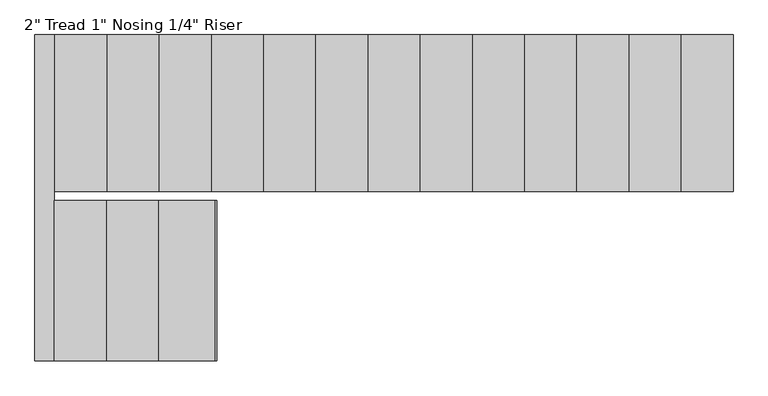
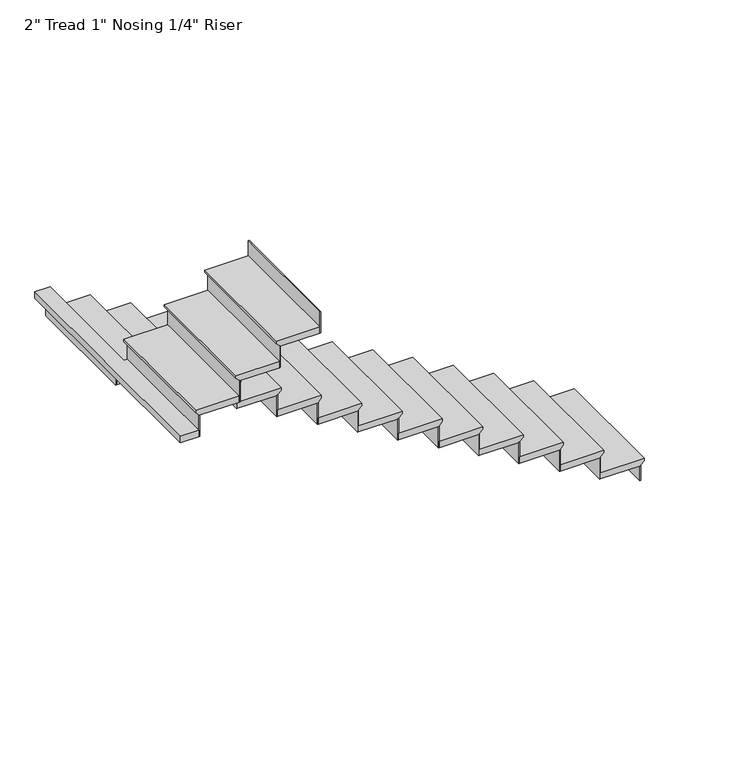
"""IFC4 building model written with IfcOpenShell, lengths in millimetres: stair flight geometry."""

from ifc_helpers import new_model, si_unit, origin, place, context, project, spatial, faceted_brep, source, transform, mapped, element, save


def stair_flight_af090c4c(model_context):
    return source(origin(), model_context, "Body", "Brep", [
        faceted_brep([(6794.5, 11386.0372886, 6246.2833333), (6794.5, 11386.0372886, 6265.3333333), (6794.5, 10471.6372886, 6265.3333333), (6794.5, 10471.6372886, 6246.2833333), (6769.1, 11386.0372886, 6220.8833333), (6769.1, 10471.6372886, 6220.8833333), (6464.3, 11386.0372886, 6265.3333333), (6464.3, 10471.6372886, 6265.3333333), (6769.1, 10471.6372886, 6214.5333333), (6464.3, 10471.6372886, 6214.5333333), (6464.3, 11386.0372886, 6214.5333333), (6769.1, 11386.0372886, 6214.5333333)], [[[0, 1, 2, 3]], [[4, 0, 3, 5]], [[2, 1, 6, 7]], [[8, 9, 10, 11]], [[2, 7, 9, 8, 5, 3]], [[8, 11, 4, 5]], [[6, 1, 0, 4, 11, 10]], [[7, 6, 10, 9]]]),
        faceted_brep([(6769.1, 11386.0372886, 6214.5333333), (6769.1, 11386.0372886, 6096.0), (6762.75, 11386.0372886, 6096.0), (6762.75, 11386.0372886, 6214.5333333), (6769.1, 10471.6372886, 6214.5333333), (6762.75, 10471.6372886, 6214.5333333), (6762.75, 10471.6372886, 6096.0), (6769.1, 10471.6372886, 6096.0)], [[[0, 1, 2, 3]], [[4, 5, 6, 7]], [[1, 0, 4, 7]], [[2, 1, 7, 6]], [[3, 2, 6, 5]], [[0, 3, 5, 4]]]),
        faceted_brep([(6464.3, 11386.0372886, 6383.8666667), (6464.3, 11386.0372886, 6214.5333333), (6457.95, 11386.0372886, 6214.5333333), (6457.95, 11386.0372886, 6383.8666667), (6464.3, 10471.6372886, 6383.8666667), (6457.95, 10471.6372886, 6383.8666667), (6457.95, 10471.6372886, 6214.5333333), (6464.3, 10471.6372886, 6214.5333333)], [[[0, 1, 2, 3]], [[4, 5, 6, 7]], [[1, 0, 4, 7]], [[2, 1, 7, 6]], [[3, 2, 6, 5]], [[0, 3, 5, 4]]]),
        faceted_brep([(6489.7, 10471.6372886, 6434.6666667), (6489.7, 11386.0372886, 6434.6666667), (6159.5, 11386.0372886, 6434.6666667), (6159.5, 10471.6372886, 6434.6666667), (6464.3, 10471.6372886, 6383.8666667), (6159.5, 10471.6372886, 6383.8666667), (6159.5, 11386.0372886, 6383.8666667), (6464.3, 11386.0372886, 6383.8666667), (6464.3, 10471.6372886, 6390.2166667), (6489.7, 10471.6372886, 6415.6166667), (6464.3, 11386.0372886, 6390.2166667), (6489.7, 11386.0372886, 6415.6166667)], [[[0, 1, 2, 3]], [[4, 5, 6, 7]], [[0, 3, 5, 4, 8, 9]], [[4, 7, 10, 8]], [[2, 1, 11, 10, 7, 6]], [[3, 2, 6, 5]], [[11, 1, 0, 9]], [[10, 11, 9, 8]]]),
        faceted_brep([(6159.5, 11386.0372886, 6553.2), (6159.5, 11386.0372886, 6383.8666667), (6153.15, 11386.0372886, 6383.8666667), (6153.15, 11386.0372886, 6553.2), (6159.5, 10471.6372886, 6553.2), (6153.15, 10471.6372886, 6553.2), (6153.15, 10471.6372886, 6383.8666667), (6159.5, 10471.6372886, 6383.8666667)], [[[0, 1, 2, 3]], [[4, 5, 6, 7]], [[1, 0, 4, 7]], [[2, 1, 7, 6]], [[3, 2, 6, 5]], [[0, 3, 5, 4]]]),
        faceted_brep([(6184.9, 10471.6372886, 6604.0), (6184.9, 11386.0372886, 6604.0), (5854.7, 11386.0372886, 6604.0), (5854.7, 10471.6372886, 6604.0), (6159.5, 10471.6372886, 6553.2), (5854.7, 10471.6372886, 6553.2), (5854.7, 11386.0372886, 6553.2), (6159.5, 11386.0372886, 6553.2), (6159.5, 10471.6372886, 6559.55), (6184.9, 10471.6372886, 6584.95), (6159.5, 11386.0372886, 6559.55), (6184.9, 11386.0372886, 6584.95)], [[[0, 1, 2, 3]], [[4, 5, 6, 7]], [[0, 3, 5, 4, 8, 9]], [[4, 7, 10, 8]], [[2, 1, 11, 10, 7, 6]], [[3, 2, 6, 5]], [[11, 1, 0, 9]], [[10, 11, 9, 8]]]),
        faceted_brep([(5854.7, 11386.0372886, 6722.5333333), (5854.7, 11386.0372886, 6553.2), (5848.35, 11386.0372886, 6553.2), (5848.35, 11386.0372886, 6722.5333333), (5854.7, 10471.6372886, 6722.5333333), (5848.35, 10471.6372886, 6722.5333333), (5848.35, 10471.6372886, 6553.2), (5854.7, 10471.6372886, 6553.2)], [[[0, 1, 2, 3]], [[4, 5, 6, 7]], [[1, 0, 4, 7]], [[2, 1, 7, 6]], [[3, 2, 6, 5]], [[0, 3, 5, 4]]]),
        faceted_brep([(5880.1, 10471.6372886, 6773.3333333), (5880.1, 11386.0372886, 6773.3333333), (5549.9, 11386.0372886, 6773.3333333), (5549.9, 10471.6372886, 6773.3333333), (5854.7, 10471.6372886, 6722.5333333), (5549.9, 10471.6372886, 6722.5333333), (5549.9, 11386.0372886, 6722.5333333), (5854.7, 11386.0372886, 6722.5333333), (5854.7, 10471.6372886, 6728.8833333), (5880.1, 10471.6372886, 6754.2833333), (5854.7, 11386.0372886, 6728.8833333), (5880.1, 11386.0372886, 6754.2833333)], [[[0, 1, 2, 3]], [[4, 5, 6, 7]], [[0, 3, 5, 4, 8, 9]], [[4, 7, 10, 8]], [[2, 1, 11, 10, 7, 6]], [[3, 2, 6, 5]], [[11, 1, 0, 9]], [[10, 11, 9, 8]]]),
        faceted_brep([(5549.9, 11386.0372886, 6891.8666667), (5549.9, 11386.0372886, 6722.5333333), (5543.55, 11386.0372886, 6722.5333333), (5543.55, 11386.0372886, 6891.8666667), (5549.9, 10471.6372886, 6891.8666667), (5543.55, 10471.6372886, 6891.8666667), (5543.55, 10471.6372886, 6722.5333333), (5549.9, 10471.6372886, 6722.5333333)], [[[0, 1, 2, 3]], [[4, 5, 6, 7]], [[1, 0, 4, 7]], [[2, 1, 7, 6]], [[3, 2, 6, 5]], [[0, 3, 5, 4]]]),
        faceted_brep([(5575.3, 10471.6372886, 6942.6666667), (5575.3, 11386.0372886, 6942.6666667), (5245.1, 11386.0372886, 6942.6666667), (5245.1, 10471.6372886, 6942.6666667), (5549.9, 10471.6372886, 6891.8666667), (5245.1, 10471.6372886, 6891.8666667), (5245.1, 11386.0372886, 6891.8666667), (5549.9, 11386.0372886, 6891.8666667), (5549.9, 10471.6372886, 6898.2166667), (5575.3, 10471.6372886, 6923.6166667), (5549.9, 11386.0372886, 6898.2166667), (5575.3, 11386.0372886, 6923.6166667)], [[[0, 1, 2, 3]], [[4, 5, 6, 7]], [[0, 3, 5, 4, 8, 9]], [[4, 7, 10, 8]], [[2, 1, 11, 10, 7, 6]], [[3, 2, 6, 5]], [[11, 1, 0, 9]], [[10, 11, 9, 8]]]),
        faceted_brep([(5245.1, 11386.0372886, 7061.2), (5245.1, 11386.0372886, 6891.8666667), (5238.75, 11386.0372886, 6891.8666667), (5238.75, 11386.0372886, 7061.2), (5245.1, 10471.6372886, 7061.2), (5238.75, 10471.6372886, 7061.2), (5238.75, 10471.6372886, 6891.8666667), (5245.1, 10471.6372886, 6891.8666667)], [[[0, 1, 2, 3]], [[4, 5, 6, 7]], [[1, 0, 4, 7]], [[2, 1, 7, 6]], [[3, 2, 6, 5]], [[0, 3, 5, 4]]]),
        faceted_brep([(5270.5, 10471.6372886, 7112.0), (5270.5, 11386.0372886, 7112.0), (4940.3, 11386.0372886, 7112.0), (4940.3, 10471.6372886, 7112.0), (5245.1, 10471.6372886, 7061.2), (4940.3, 10471.6372886, 7061.2), (4940.3, 11386.0372886, 7061.2), (5245.1, 11386.0372886, 7061.2), (5245.1, 10471.6372886, 7067.55), (5270.5, 10471.6372886, 7092.95), (5245.1, 11386.0372886, 7067.55), (5270.5, 11386.0372886, 7092.95)], [[[0, 1, 2, 3]], [[4, 5, 6, 7]], [[0, 3, 5, 4, 8, 9]], [[4, 7, 10, 8]], [[2, 1, 11, 10, 7, 6]], [[3, 2, 6, 5]], [[11, 1, 0, 9]], [[10, 11, 9, 8]]]),
        faceted_brep([(4940.3, 11386.0372886, 7230.5333333), (4940.3, 11386.0372886, 7061.2), (4933.95, 11386.0372886, 7061.2), (4933.95, 11386.0372886, 7230.5333333), (4940.3, 10471.6372886, 7230.5333333), (4933.95, 10471.6372886, 7230.5333333), (4933.95, 10471.6372886, 7061.2), (4940.3, 10471.6372886, 7061.2)], [[[0, 1, 2, 3]], [[4, 5, 6, 7]], [[1, 0, 4, 7]], [[2, 1, 7, 6]], [[3, 2, 6, 5]], [[0, 3, 5, 4]]]),
        faceted_brep([(4965.7, 10471.6372886, 7281.3333333), (4965.7, 11386.0372886, 7281.3333333), (4635.5, 11386.0372886, 7281.3333333), (4635.5, 10471.6372886, 7281.3333333), (4940.3, 10471.6372886, 7230.5333333), (4635.5, 10471.6372886, 7230.5333333), (4635.5, 11386.0372886, 7230.5333333), (4940.3, 11386.0372886, 7230.5333333), (4940.3, 10471.6372886, 7236.8833333), (4965.7, 10471.6372886, 7262.2833333), (4940.3, 11386.0372886, 7236.8833333), (4965.7, 11386.0372886, 7262.2833333)], [[[0, 1, 2, 3]], [[4, 5, 6, 7]], [[0, 3, 5, 4, 8, 9]], [[4, 7, 10, 8]], [[2, 1, 11, 10, 7, 6]], [[3, 2, 6, 5]], [[11, 1, 0, 9]], [[10, 11, 9, 8]]]),
        faceted_brep([(4635.5, 11386.0372886, 7399.8666667), (4635.5, 11386.0372886, 7230.5333333), (4629.15, 11386.0372886, 7230.5333333), (4629.15, 11386.0372886, 7399.8666667), (4635.5, 10471.6372886, 7399.8666667), (4629.15, 10471.6372886, 7399.8666667), (4629.15, 10471.6372886, 7230.5333333), (4635.5, 10471.6372886, 7230.5333333)], [[[0, 1, 2, 3]], [[4, 5, 6, 7]], [[1, 0, 4, 7]], [[2, 1, 7, 6]], [[3, 2, 6, 5]], [[0, 3, 5, 4]]]),
        faceted_brep([(4660.9, 10471.6372886, 7450.6666667), (4660.9, 11386.0372886, 7450.6666667), (4330.7, 11386.0372886, 7450.6666667), (4330.7, 10471.6372886, 7450.6666667), (4635.5, 10471.6372886, 7399.8666667), (4330.7, 10471.6372886, 7399.8666667), (4330.7, 11386.0372886, 7399.8666667), (4635.5, 11386.0372886, 7399.8666667), (4635.5, 10471.6372886, 7406.2166667), (4660.9, 10471.6372886, 7431.6166667), (4635.5, 11386.0372886, 7406.2166667), (4660.9, 11386.0372886, 7431.6166667)], [[[0, 1, 2, 3]], [[4, 5, 6, 7]], [[0, 3, 5, 4, 8, 9]], [[4, 7, 10, 8]], [[2, 1, 11, 10, 7, 6]], [[3, 2, 6, 5]], [[11, 1, 0, 9]], [[10, 11, 9, 8]]]),
        faceted_brep([(4330.7, 11386.0372886, 7569.2), (4330.7, 11386.0372886, 7399.8666667), (4324.35, 11386.0372886, 7399.8666667), (4324.35, 11386.0372886, 7569.2), (4330.7, 10471.6372886, 7569.2), (4324.35, 10471.6372886, 7569.2), (4324.35, 10471.6372886, 7399.8666667), (4330.7, 10471.6372886, 7399.8666667)], [[[0, 1, 2, 3]], [[4, 5, 6, 7]], [[1, 0, 4, 7]], [[2, 1, 7, 6]], [[3, 2, 6, 5]], [[0, 3, 5, 4]]]),
        faceted_brep([(4356.1, 10471.6372886, 7620.0), (4356.1, 11386.0372886, 7620.0), (4025.9, 11386.0372886, 7620.0), (4025.9, 10471.6372886, 7620.0), (4330.7, 10471.6372886, 7569.2), (4025.9, 10471.6372886, 7569.2), (4025.9, 11386.0372886, 7569.2), (4330.7, 11386.0372886, 7569.2), (4330.7, 10471.6372886, 7575.55), (4356.1, 10471.6372886, 7600.95), (4330.7, 11386.0372886, 7575.55), (4356.1, 11386.0372886, 7600.95)], [[[0, 1, 2, 3]], [[4, 5, 6, 7]], [[0, 3, 5, 4, 8, 9]], [[4, 7, 10, 8]], [[2, 1, 11, 10, 7, 6]], [[3, 2, 6, 5]], [[11, 1, 0, 9]], [[10, 11, 9, 8]]]),
        faceted_brep([(4025.9, 11386.0372886, 7738.5333333), (4025.9, 11386.0372886, 7569.2), (4019.55, 11386.0372886, 7569.2), (4019.55, 11386.0372886, 7738.5333333), (4025.9, 10471.6372886, 7738.5333333), (4019.55, 10471.6372886, 7738.5333333), (4019.55, 10471.6372886, 7569.2), (4025.9, 10471.6372886, 7569.2)], [[[0, 1, 2, 3]], [[4, 5, 6, 7]], [[1, 0, 4, 7]], [[2, 1, 7, 6]], [[3, 2, 6, 5]], [[0, 3, 5, 4]]]),
        faceted_brep([(4051.3, 10471.6372886, 7789.3333333), (4051.3, 11386.0372886, 7789.3333333), (3721.1, 11386.0372886, 7789.3333333), (3721.1, 10471.6372886, 7789.3333333), (4025.9, 10471.6372886, 7738.5333333), (3721.1, 10471.6372886, 7738.5333333), (3721.1, 11386.0372886, 7738.5333333), (4025.9, 11386.0372886, 7738.5333333), (4025.9, 10471.6372886, 7744.8833333), (4051.3, 10471.6372886, 7770.2833333), (4025.9, 11386.0372886, 7744.8833333), (4051.3, 11386.0372886, 7770.2833333)], [[[0, 1, 2, 3]], [[4, 5, 6, 7]], [[0, 3, 5, 4, 8, 9]], [[4, 7, 10, 8]], [[2, 1, 11, 10, 7, 6]], [[3, 2, 6, 5]], [[11, 1, 0, 9]], [[10, 11, 9, 8]]]),
        faceted_brep([(3721.1, 11386.0372886, 7907.8666667), (3721.1, 11386.0372886, 7738.5333333), (3714.75, 11386.0372886, 7738.5333333), (3714.75, 11386.0372886, 7907.8666667), (3721.1, 10471.6372886, 7907.8666667), (3714.75, 10471.6372886, 7907.8666667), (3714.75, 10471.6372886, 7738.5333333), (3721.1, 10471.6372886, 7738.5333333)], [[[0, 1, 2, 3]], [[4, 5, 6, 7]], [[1, 0, 4, 7]], [[2, 1, 7, 6]], [[3, 2, 6, 5]], [[0, 3, 5, 4]]]),
        faceted_brep([(3746.5, 10471.6372886, 7958.6666667), (3746.5, 11386.0372886, 7958.6666667), (3416.3, 11386.0372886, 7958.6666667), (3416.3, 10471.6372886, 7958.6666667), (3721.1, 10471.6372886, 7907.8666667), (3416.3, 10471.6372886, 7907.8666667), (3416.3, 11386.0372886, 7907.8666667), (3721.1, 11386.0372886, 7907.8666667), (3721.1, 10471.6372886, 7914.2166667), (3746.5, 10471.6372886, 7939.6166667), (3721.1, 11386.0372886, 7914.2166667), (3746.5, 11386.0372886, 7939.6166667)], [[[0, 1, 2, 3]], [[4, 5, 6, 7]], [[0, 3, 5, 4, 8, 9]], [[4, 7, 10, 8]], [[2, 1, 11, 10, 7, 6]], [[3, 2, 6, 5]], [[11, 1, 0, 9]], [[10, 11, 9, 8]]]),
        faceted_brep([(3416.3, 11386.0372886, 8077.2), (3416.3, 11386.0372886, 7907.8666667), (3409.95, 11386.0372886, 7907.8666667), (3409.95, 11386.0372886, 8077.2), (3416.3, 10471.6372886, 8077.2), (3409.95, 10471.6372886, 8077.2), (3409.95, 10471.6372886, 7907.8666667), (3416.3, 10471.6372886, 7907.8666667)], [[[0, 1, 2, 3]], [[4, 5, 6, 7]], [[1, 0, 4, 7]], [[2, 1, 7, 6]], [[3, 2, 6, 5]], [[0, 3, 5, 4]]]),
        faceted_brep([(3441.7, 10471.6372886, 8128.0), (3441.7, 11386.0372886, 8128.0), (3111.5, 11386.0372886, 8128.0), (3111.5, 10471.6372886, 8128.0), (3416.3, 10471.6372886, 8077.2), (3111.5, 10471.6372886, 8077.2), (3111.5, 11386.0372886, 8077.2), (3416.3, 11386.0372886, 8077.2), (3416.3, 10471.6372886, 8083.55), (3441.7, 10471.6372886, 8108.95), (3416.3, 11386.0372886, 8083.55), (3441.7, 11386.0372886, 8108.95)], [[[0, 1, 2, 3]], [[4, 5, 6, 7]], [[0, 3, 5, 4, 8, 9]], [[4, 7, 10, 8]], [[2, 1, 11, 10, 7, 6]], [[3, 2, 6, 5]], [[11, 1, 0, 9]], [[10, 11, 9, 8]]]),
        faceted_brep([(3111.5, 11386.0372886, 8246.5333333), (3111.5, 11386.0372886, 8077.2), (3105.15, 11386.0372886, 8077.2), (3105.15, 11386.0372886, 8246.5333333), (3111.5, 10471.6372886, 8246.5333333), (3105.15, 10471.6372886, 8246.5333333), (3105.15, 10471.6372886, 8077.2), (3111.5, 10471.6372886, 8077.2)], [[[0, 1, 2, 3]], [[4, 5, 6, 7]], [[1, 0, 4, 7]], [[2, 1, 7, 6]], [[3, 2, 6, 5]], [[0, 3, 5, 4]]]),
        faceted_brep([(3136.9, 10471.6372886, 8297.3333333), (3136.9, 11386.0372886, 8297.3333333), (2806.7, 11386.0372886, 8297.3333333), (2806.7, 10471.6372886, 8297.3333333), (3111.5, 10471.6372886, 8246.5333333), (2806.7, 10471.6372886, 8246.5333333), (2806.7, 11386.0372886, 8246.5333333), (3111.5, 11386.0372886, 8246.5333333), (3111.5, 10471.6372886, 8252.8833333), (3136.9, 10471.6372886, 8278.2833333), (3111.5, 11386.0372886, 8252.8833333), (3136.9, 11386.0372886, 8278.2833333)], [[[0, 1, 2, 3]], [[4, 5, 6, 7]], [[0, 3, 5, 4, 8, 9]], [[4, 7, 10, 8]], [[2, 1, 11, 10, 7, 6]], [[3, 2, 6, 5]], [[11, 1, 0, 9]], [[10, 11, 9, 8]]]),
        faceted_brep([(2806.7, 11386.0372886, 8415.8666667), (2806.7, 11386.0372886, 8246.5333333), (2800.35, 11386.0372886, 8246.5333333), (2800.35, 11386.0372886, 8415.8666667), (2806.7, 10471.6372886, 8415.8666667), (2800.35, 10471.6372886, 8415.8666667), (2800.35, 10471.6372886, 8246.5333333), (2806.7, 10471.6372886, 8246.5333333)], [[[0, 1, 2, 3]], [[4, 5, 6, 7]], [[1, 0, 4, 7]], [[2, 1, 7, 6]], [[3, 2, 6, 5]], [[0, 3, 5, 4]]]),
        faceted_brep([(2857.5, 10418.2972886, 8466.6666667), (2832.1, 10418.2972886, 8466.6666667), (2832.1, 11386.0372886, 8466.6666667), (2717.8, 11386.0372886, 8466.6666667), (2717.8, 9481.0372886, 8466.6666667), (2857.5, 9481.0372886, 8466.6666667), (2832.1, 10418.2972886, 8415.8666667), (2857.5, 10418.2972886, 8415.8666667), (2857.5, 9481.0372886, 8415.8666667), (2717.8, 9481.0372886, 8415.8666667), (2717.8, 11386.0372886, 8415.8666667), (2806.7, 11386.0372886, 8415.8666667), (2806.7, 10471.6372886, 8415.8666667), (2832.1, 10471.6372886, 8415.8666667), (2832.1, 10471.6372886, 8447.6166667), (2832.1, 11386.0372886, 8447.6166667), (2806.7, 10471.6372886, 8422.2166667), (2806.7, 11386.0372886, 8422.2166667)], [[[0, 1, 2, 3, 4, 5]], [[6, 7, 8, 9, 10, 11, 12, 13]], [[1, 0, 7, 6]], [[2, 1, 6, 13, 14, 15]], [[13, 12, 16, 14]], [[12, 11, 17, 16]], [[3, 2, 15, 17, 11, 10]], [[4, 3, 10, 9]], [[5, 4, 9, 8]], [[0, 5, 8, 7]], [[17, 15, 14, 16]]]),
        faceted_brep([(2857.5, 9481.0372886, 8585.2), (2857.5, 9481.0372886, 8415.8666667), (2863.85, 9481.0372886, 8415.8666667), (2863.85, 9481.0372886, 8585.2), (2857.5, 10418.2972886, 8585.2), (2863.85, 10418.2972886, 8585.2), (2863.85, 10418.2972886, 8415.8666667), (2857.5, 10418.2972886, 8415.8666667)], [[[0, 1, 2, 3]], [[4, 5, 6, 7]], [[1, 0, 4, 7]], [[2, 1, 7, 6]], [[3, 2, 6, 5]], [[0, 3, 5, 4]]]),
        faceted_brep([(2832.1, 10418.2972886, 8636.0), (2832.1, 9481.0372886, 8636.0), (3162.3, 9481.0372886, 8636.0), (3162.3, 10418.2972886, 8636.0), (2857.5, 10418.2972886, 8585.2), (3162.3, 10418.2972886, 8585.2), (3162.3, 9481.0372886, 8585.2), (2857.5, 9481.0372886, 8585.2), (2857.5, 10418.2972886, 8591.55), (2832.1, 10418.2972886, 8616.95), (2857.5, 9481.0372886, 8591.55), (2832.1, 9481.0372886, 8616.95)], [[[0, 1, 2, 3]], [[4, 5, 6, 7]], [[0, 3, 5, 4, 8, 9]], [[4, 7, 10, 8]], [[2, 1, 11, 10, 7, 6]], [[3, 2, 6, 5]], [[11, 1, 0, 9]], [[10, 11, 9, 8]]]),
        faceted_brep([(3162.3, 9481.0372886, 8754.5333333), (3162.3, 9481.0372886, 8585.2), (3168.65, 9481.0372886, 8585.2), (3168.65, 9481.0372886, 8754.5333333), (3162.3, 10418.2972886, 8754.5333333), (3168.65, 10418.2972886, 8754.5333333), (3168.65, 10418.2972886, 8585.2), (3162.3, 10418.2972886, 8585.2)], [[[0, 1, 2, 3]], [[4, 5, 6, 7]], [[1, 0, 4, 7]], [[2, 1, 7, 6]], [[3, 2, 6, 5]], [[0, 3, 5, 4]]]),
        faceted_brep([(3136.9, 10418.2972886, 8805.3333333), (3136.9, 9481.0372886, 8805.3333333), (3467.1, 9481.0372886, 8805.3333333), (3467.1, 10418.2972886, 8805.3333333), (3162.3, 10418.2972886, 8754.5333333), (3467.1, 10418.2972886, 8754.5333333), (3467.1, 9481.0372886, 8754.5333333), (3162.3, 9481.0372886, 8754.5333333), (3162.3, 10418.2972886, 8760.8833333), (3136.9, 10418.2972886, 8786.2833333), (3162.3, 9481.0372886, 8760.8833333), (3136.9, 9481.0372886, 8786.2833333)], [[[0, 1, 2, 3]], [[4, 5, 6, 7]], [[0, 3, 5, 4, 8, 9]], [[4, 7, 10, 8]], [[2, 1, 11, 10, 7, 6]], [[3, 2, 6, 5]], [[11, 1, 0, 9]], [[10, 11, 9, 8]]]),
        faceted_brep([(3467.1, 9481.0372886, 8923.8666667), (3467.1, 9481.0372886, 8754.5333333), (3473.45, 9481.0372886, 8754.5333333), (3473.45, 9481.0372886, 8923.8666667), (3467.1, 10418.2972886, 8923.8666667), (3473.45, 10418.2972886, 8923.8666667), (3473.45, 10418.2972886, 8754.5333333), (3467.1, 10418.2972886, 8754.5333333)], [[[0, 1, 2, 3]], [[4, 5, 6, 7]], [[1, 0, 4, 7]], [[2, 1, 7, 6]], [[3, 2, 6, 5]], [[0, 3, 5, 4]]]),
        faceted_brep([(3771.9019847, 9481.0372886, 9093.2), (3771.9019847, 9481.0372886, 8923.8666667), (3778.2519847, 9481.0372886, 8923.8666667), (3778.2519847, 9481.0372886, 9093.2), (3771.9019847, 10418.2972886, 9093.2), (3778.2519847, 10418.2972886, 9093.2), (3778.2519847, 10418.2972886, 8923.8666667), (3771.9019847, 10418.2972886, 8923.8666667)], [[[0, 1, 2, 3]], [[4, 5, 6, 7]], [[1, 0, 4, 7]], [[2, 1, 7, 6]], [[3, 2, 6, 5]], [[0, 3, 5, 4]]]),
        faceted_brep([(3441.7, 10418.2972886, 8974.6666667), (3441.7, 9481.0372886, 8974.6666667), (3771.9019847, 9481.0372886, 8974.6666667), (3771.9019847, 10418.2972886, 8974.6666667), (3467.1, 10418.2972886, 8923.8666667), (3771.9019847, 10418.2972886, 8923.8666667), (3771.9019847, 9481.0372886, 8923.8666667), (3467.1, 9481.0372886, 8923.8666667), (3467.1, 10418.2972886, 8930.2166667), (3441.7, 10418.2972886, 8955.6166667), (3467.1, 9481.0372886, 8930.2166667), (3441.7, 9481.0372886, 8955.6166667)], [[[0, 1, 2, 3]], [[4, 5, 6, 7]], [[0, 3, 5, 4, 8, 9]], [[4, 7, 10, 8]], [[2, 1, 11, 10, 7, 6]], [[3, 2, 6, 5]], [[11, 1, 0, 9]], [[10, 11, 9, 8]]]),
    ])


if __name__ == "__main__":
    model = new_model("IFC4")
    model_context = context("Model", 3, world=origin())
    ifc_project = project(units=[si_unit("LENGTHUNIT", "METRE", prefix="MILLI")], contexts=[model_context])
    site = spatial("IfcSite", under=ifc_project)
    building = spatial("IfcBuilding", under=site)
    placement = place(None, origin())
    stair_flight_shape = stair_flight_af090c4c(model_context)
    element("IfcStairFlight", 1, ObjectType="2\" Tread 1\" Nosing 1/4\" Riser", at=placement, inside=building, context=model_context, shape_type="MappedRepresentation", body=[
        mapped(stair_flight_shape, transform((0.0, 0.0, 0.0), x_axis=(1.0, 0.0, 0.0), y_axis=(0.0, 1.0, 0.0), z_axis=(0.0, 0.0, 1.0))),
    ])
    save(model, "model.ifc")
